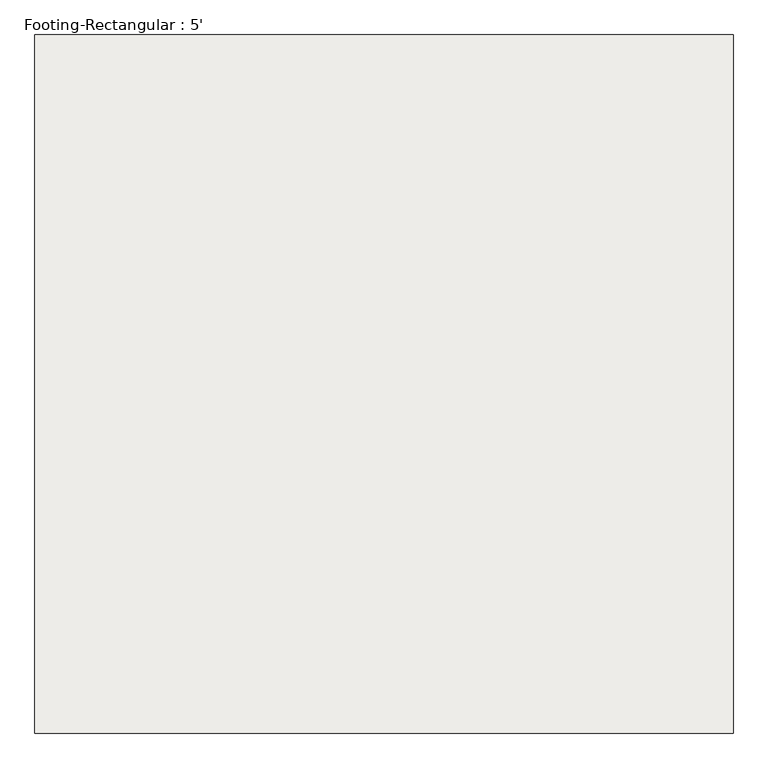
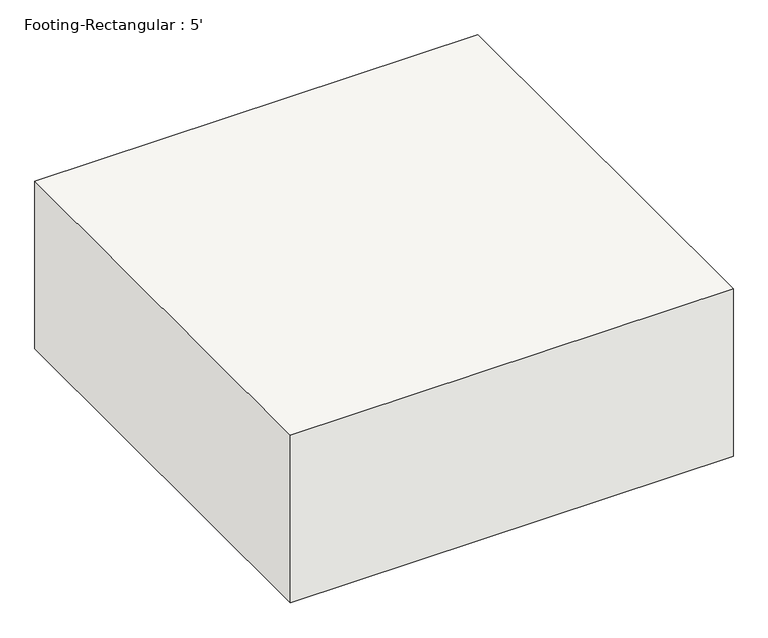
"""IFC4 building model written with IfcOpenShell, lengths in millimetres: slab geometry, Footing-Rectangular : 5'."""

from ifc_helpers import new_model, si_unit, frame, origin, place, context, project, spatial, polyline, outline, extrude, source, transform, mapped, element, save


def footing_rectangular_5_c859e583(model_context):
    return source(origin(), model_context, "Body", "SweptSolid", [
        extrude(outline(polyline([(762.0, 762.0), (762.0, -762.0), (-762.0, -762.0), (-762.0, 762.0), (762.0, 762.0)])), frame((0.0, 0.0, -609.6), z_axis=(0.0, 0.0, 1.0), x_axis=(1.0, 0.0, 0.0)), (0.0, 0.0, 1.0), 609.6),
    ])


if __name__ == "__main__":
    model = new_model("IFC4")
    model_context = context("Model", 3, world=origin())
    ifc_project = project(units=[si_unit("LENGTHUNIT", "METRE", prefix="MILLI")], contexts=[model_context])
    site = spatial("IfcSite", under=ifc_project)
    building = spatial("IfcBuilding", under=site)
    placement = place(None, origin())
    footing_rectangular_5_shape = footing_rectangular_5_c859e583(model_context)
    element("IfcSlab", 1, ObjectType="Footing-Rectangular : 5'", at=placement, inside=building, context=model_context, shape_type="MappedRepresentation", body=[
        mapped(footing_rectangular_5_shape, transform((0.0, 0.0, 0.0), x_axis=(1.0, 0.0, 0.0), y_axis=(0.0, 1.0, 0.0), z_axis=(0.0, 0.0, 1.0))),
    ])
    save(model, "model.ifc")

# Revit data of these elements
# Type "Footing-Rectangular : 5'"
#   Assembly Code = "A1010100"
#   Width = 5' - 0"
#   Length = 5' - 0"
#   Foundation Thickness = 2' - 0"
#   Structural Material [instance default] = Concrete, Cast-in-Place gray
# Element 1 (IfcSlab, "Footing-Rectangular : 5'")
#   Materials on its faces: "Concrete, Cast-in-Place gray"
# Materials
#   "Concrete, Cast-in-Place gray": class "Concrete", colour RGB 192 192 192, transparency 0, Description = "Cast-in-place concrete", Cost = 0
